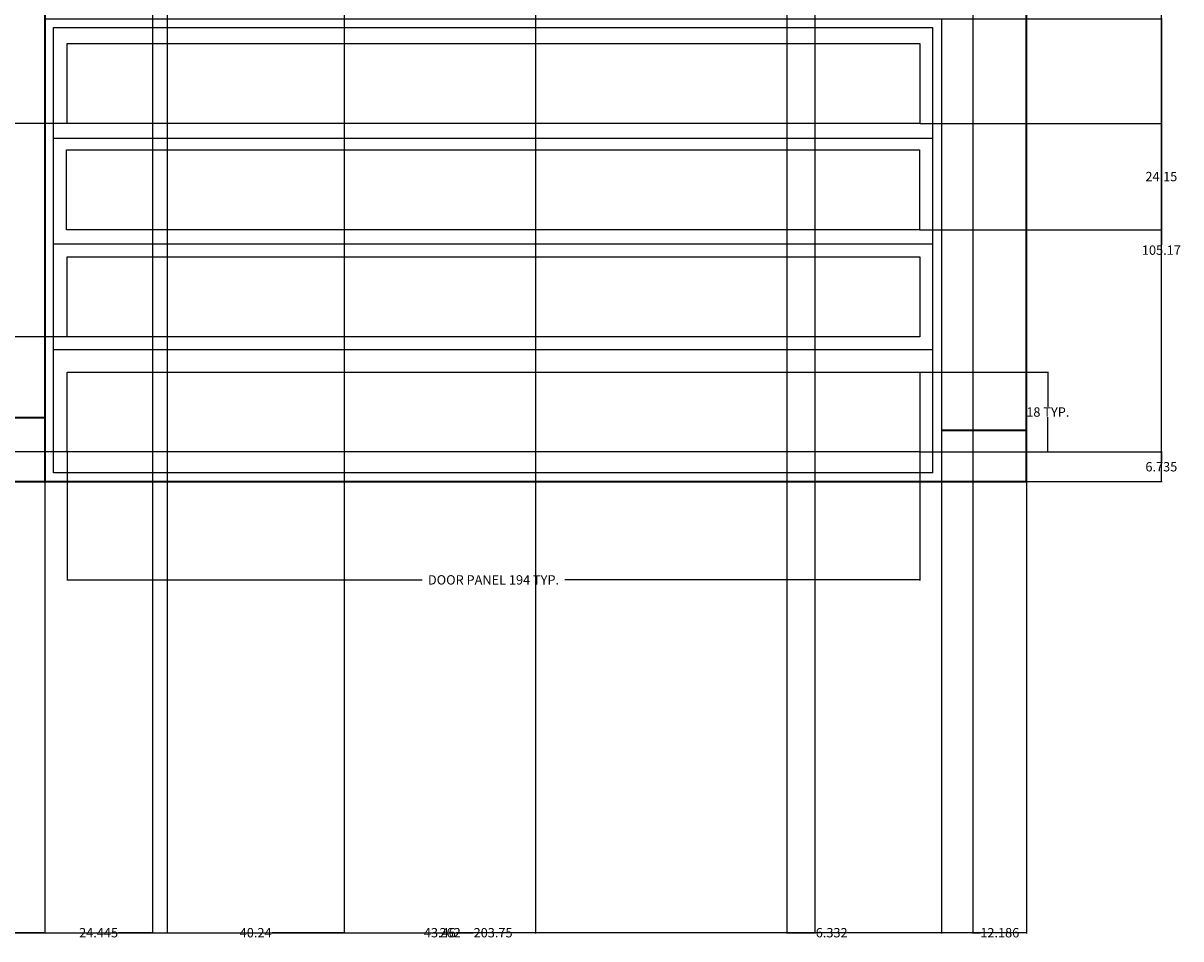
# Model space of a CAD drawing. Units: inches. Extents: x -113 to 379, y 13 to 689.
# Tile 2 of 5: x 116 to 379, y 13 to 221. Entities that reach past the tile are written whole.
import ezdxf

# ---------------------------------------------------------------- set-up
doc = ezdxf.new("R2010")
doc.units = ezdxf.units.IN
doc.header["$MEASUREMENT"] = 0
for name, color, linetype, lineweight in [('A-ANNO-DIMS', 2, 'Continuous', 18), ('A-DOOR', 3, 'Continuous', 25), ('A-WALL', 7, 'Continuous', 35), ('C-TOPO', 8, 'Continuous', 35)]:
    doc.layers.add(name, color=color, linetype=linetype, lineweight=lineweight)
doc.styles.get("Standard").update_dxf_attribs({"font": 'arial.ttf'})
doc.dimstyles.get("Standard").update_dxf_attribs({"dimtxt": 2.125, "dimasz": 0.18, "dimexe": 0.18, "dimexo": 0.0625, "dimgap": 0.09, "dimtad": 0, "dimtih": 1, "dimtoh": 1, "dimdec": 4, "dimzin": 0, "dimdsep": 46, "dimlunit": 4, "dimtxsty": 'Standard', "dimcen": 0.09, "dimadec": 0, "dimazin": 0, "dimtfac": 1, "dimtdec": 4, "dimtofl": 0, "dimtmove": 0, "dimatfit": 3, "dimfxl": 1, "dimtolj": 1, "dimtzin": 0, "dimarcsym": 0})

# ---------------------------------------------------------------- blocks, each defined once
blk = doc.blocks.new('GARAGE-DOOR-PANEL')
blk.add_lwpolyline([(0, 18.13), (193.81, 18.13), (193.81, 0), (0, 0)], close=True)
blk = doc.blocks.new('*D11')
at = {"layer": 'A-ANNO-DIMS', "color": 0, "lineweight": -2, "transparency": 16777216}
for p, q in [((125.81, 123.32), (125.81, 94.13)), ((319.62, 123.32), (319.62, 94.13)), ((125.99, 94.31), (206.54, 94.31)), ((319.44, 94.31), (238.9, 94.31))]:
    blk.add_line(p, q, dxfattribs=at)
at = {"layer": 'A-ANNO-DIMS', "color": 0, "transparency": 16777216}
for points in [[(125.99, 94.34), (125.99, 94.28), (125.81, 94.31)], [(319.44, 94.34), (319.44, 94.28), (319.62, 94.31)]]:
    blk.add_solid(points, dxfattribs=at)
at = {"layer": 'Defpoints', "color": 0, "transparency": 16777216}
for p in [(125.81, 123.39), (319.62, 123.39), (319.62, 94.31)]:
    blk.add_point(p, dxfattribs=at)
at = {"layer": 'A-ANNO-DIMS', "color": 0, "transparency": 16777216, "insert": (222.72, 94.31), "char_height": 2.125, "attachment_point": 5}
blk.add_mtext('\\A1;DOOR PANEL 194 TYP.', dxfattribs=at)
blk = doc.blocks.new('*D12')
at = {"layer": 'A-ANNO-DIMS', "color": 0, "lineweight": -2, "transparency": 16777216}
for p, q in [((319.69, 141.52), (348.88, 141.52)), ((348.7, 141.34), (348.7, 133.63)), ((348.7, 123.57), (348.7, 131.28)), ((319.69, 123.39), (348.88, 123.39))]:
    blk.add_line(p, q, dxfattribs=at)
at = {"layer": 'A-ANNO-DIMS', "color": 0, "transparency": 16777216}
for points in [[(348.67, 141.34), (348.73, 141.34), (348.7, 141.52)], [(348.67, 123.57), (348.73, 123.57), (348.7, 123.39)]]:
    blk.add_solid(points, dxfattribs=at)
at = {"layer": 'Defpoints', "color": 0, "transparency": 16777216}
for p in [(319.62, 141.52), (348.7, 141.52), (319.62, 123.39)]:
    blk.add_point(p, dxfattribs=at)
at = {"layer": 'A-ANNO-DIMS', "color": 0, "transparency": 16777216, "insert": (348.7, 132.45), "char_height": 2.125, "attachment_point": 5}
blk.add_mtext('\\A1;18 TYP.', dxfattribs=at)
blk = doc.blocks.new('*D19')
at = {"layer": 'A-ANNO-DIMS', "color": 0, "lineweight": -2, "transparency": 16777216}
for p, q in [((81.87, 116.59), (81.87, 13.95)), ((343.87, 116.59), (343.87, 13.95)), ((82.05, 14.13), (210.43, 14.13)), ((343.69, 14.13), (215.32, 14.13))]:
    blk.add_line(p, q, dxfattribs=at)
at = {"layer": 'A-ANNO-DIMS', "color": 0, "transparency": 16777216}
for points in [[(82.05, 14.16), (82.05, 14.1), (81.87, 14.13)], [(343.69, 14.16), (343.69, 14.1), (343.87, 14.13)]]:
    blk.add_solid(points, dxfattribs=at)
at = {"layer": 'Defpoints', "color": 0, "transparency": 16777216}
for p in [(81.87, 116.65), (343.87, 116.65), (343.87, 14.13)]:
    blk.add_point(p, dxfattribs=at)
at = {"layer": 'A-ANNO-DIMS', "color": 0, "transparency": 16777216, "insert": (212.87, 14.13), "char_height": 2.125, "attachment_point": 5}
blk.add_mtext('\\A1;262', dxfattribs=at)
blk = doc.blocks.new('*D20')
at = {"layer": 'A-ANNO-DIMS', "color": 0, "lineweight": -2, "transparency": 16777216}
for p, q in [((232.74, 657.3), (374.68, 657.3)), ((374.5, 657.12), (374.5, 388.15)), ((374.5, 116.83), (374.5, 385.8)), ((343.93, 116.65), (374.68, 116.65))]:
    blk.add_line(p, q, dxfattribs=at)
at = {"layer": 'A-ANNO-DIMS', "color": 0, "transparency": 16777216}
for points in [[(374.47, 657.12), (374.53, 657.12), (374.5, 657.3)], [(374.47, 116.83), (374.53, 116.83), (374.5, 116.65)]]:
    blk.add_solid(points, dxfattribs=at)
at = {"layer": 'Defpoints', "color": 0, "transparency": 16777216}
for p in [(232.68, 657.3), (374.5, 657.3), (343.87, 116.65)]:
    blk.add_point(p, dxfattribs=at)
at = {"layer": 'A-ANNO-DIMS', "color": 0, "transparency": 16777216, "insert": (374.5, 386.98), "char_height": 2.125, "attachment_point": 5}
blk.add_mtext('\\A1;540.7', dxfattribs=at)
blk = doc.blocks.new('*D34')
at = {"layer": 'A-ANNO-DIMS', "color": 0, "lineweight": -2, "transparency": 16777216}
for p, q in [((120.75, 116.59), (120.75, 13.95)), ((324.51, 116.59), (324.51, 13.95)), ((120.93, 14.13), (218.1, 14.13)), ((324.33, 14.13), (227.16, 14.13))]:
    blk.add_line(p, q, dxfattribs=at)
at = {"layer": 'A-ANNO-DIMS', "color": 0, "transparency": 16777216}
for points in [[(120.93, 14.16), (120.93, 14.1), (120.75, 14.13)], [(324.33, 14.16), (324.33, 14.1), (324.51, 14.13)]]:
    blk.add_solid(points, dxfattribs=at)
at = {"layer": 'Defpoints', "color": 0, "transparency": 16777216}
for p in [(120.75, 116.65), (324.51, 116.65), (324.51, 14.13)]:
    blk.add_point(p, dxfattribs=at)
at = {"layer": 'A-ANNO-DIMS', "color": 0, "transparency": 16777216, "insert": (222.63, 14.13), "char_height": 2.125, "attachment_point": 5}
blk.add_mtext('\\A1;203.75', dxfattribs=at)
blk = doc.blocks.new('*D35')
at = {"layer": 'A-ANNO-DIMS', "color": 0, "lineweight": -2, "transparency": 16777216}
for p, q in [((324.57, 221.82), (374.68, 221.82)), ((374.5, 221.64), (374.5, 170.41)), ((374.5, 116.83), (374.5, 168.06)), ((324.57, 116.65), (374.68, 116.65))]:
    blk.add_line(p, q, dxfattribs=at)
at = {"layer": 'A-ANNO-DIMS', "color": 0, "transparency": 16777216}
for points in [[(374.47, 221.64), (374.53, 221.64), (374.5, 221.82)], [(374.47, 116.83), (374.53, 116.83), (374.5, 116.65)]]:
    blk.add_solid(points, dxfattribs=at)
at = {"layer": 'Defpoints', "color": 0, "transparency": 16777216}
for p in [(324.51, 221.82), (374.5, 221.82), (324.51, 116.65)]:
    blk.add_point(p, dxfattribs=at)
at = {"layer": 'A-ANNO-DIMS', "color": 0, "transparency": 16777216, "insert": (374.5, 169.24), "char_height": 2.125, "attachment_point": 5}
blk.add_mtext('\\A1;105.17', dxfattribs=at)
blk = doc.blocks.new('*D37')
at = {"layer": 'A-ANNO-DIMS', "color": 0, "lineweight": -2, "transparency": 16777216}
for p, q in [((99.93, 116.59), (99.93, 13.95)), ((120.75, 116.59), (120.75, 13.95)), ((100.11, 14.13), (106.66, 14.13)), ((120.57, 14.13), (114.03, 14.13))]:
    blk.add_line(p, q, dxfattribs=at)
at = {"layer": 'A-ANNO-DIMS', "color": 0, "transparency": 16777216}
for points in [[(100.11, 14.16), (100.11, 14.1), (99.93, 14.13)], [(120.57, 14.16), (120.57, 14.1), (120.75, 14.13)]]:
    blk.add_solid(points, dxfattribs=at)
at = {"layer": 'Defpoints', "color": 0, "transparency": 16777216}
for p in [(99.93, 116.65), (120.75, 116.65), (120.75, 14.13)]:
    blk.add_point(p, dxfattribs=at)
at = {"layer": 'A-ANNO-DIMS', "color": 0, "transparency": 16777216, "insert": (110.34, 14.13), "char_height": 2.125, "attachment_point": 5}
blk.add_mtext('\\A1;20.82', dxfattribs=at)
blk = doc.blocks.new('*D41')
at = {"layer": 'A-ANNO-DIMS', "color": 0, "lineweight": -2, "transparency": 16777216}
for p, q in [((120.75, 286.39), (120.75, 13.95)), ((145.2, 286.39), (145.2, 13.95)), ((120.93, 14.13), (128.45, 14.13)), ((145.02, 14.13), (137.5, 14.13))]:
    blk.add_line(p, q, dxfattribs=at)
at = {"layer": 'A-ANNO-DIMS', "color": 0, "transparency": 16777216}
for points in [[(120.93, 14.16), (120.93, 14.1), (120.75, 14.13)], [(145.02, 14.16), (145.02, 14.1), (145.2, 14.13)]]:
    blk.add_solid(points, dxfattribs=at)
at = {"layer": 'Defpoints', "color": 0, "transparency": 16777216}
for p in [(120.75, 286.45), (145.2, 286.45), (145.2, 14.13)]:
    blk.add_point(p, dxfattribs=at)
at = {"layer": 'A-ANNO-DIMS', "color": 0, "transparency": 16777216, "insert": (132.98, 14.13), "char_height": 2.125, "attachment_point": 5}
blk.add_mtext('\\A1;24.445', dxfattribs=at)
blk = doc.blocks.new('*D44')
at = {"layer": 'A-ANNO-DIMS', "color": 0, "lineweight": -2, "transparency": 16777216}
for p, q in [((331.68, 303.98), (331.68, 13.95)), ((343.87, 260.59), (343.87, 13.95)), ((331.86, 14.13), (333.38, 14.13)), ((343.69, 14.13), (342.18, 14.13))]:
    blk.add_line(p, q, dxfattribs=at)
at = {"layer": 'A-ANNO-DIMS', "color": 0, "transparency": 16777216}
for points in [[(331.86, 14.16), (331.86, 14.1), (331.68, 14.13)], [(343.69, 14.16), (343.69, 14.1), (343.87, 14.13)]]:
    blk.add_solid(points, dxfattribs=at)
at = {"layer": 'Defpoints', "color": 0, "transparency": 16777216}
for p in [(331.68, 304.04), (343.87, 260.65), (343.87, 14.13)]:
    blk.add_point(p, dxfattribs=at)
at = {"layer": 'A-ANNO-DIMS', "color": 0, "transparency": 16777216, "insert": (337.78, 14.13), "char_height": 2.125, "attachment_point": 5}
blk.add_mtext('\\A1;12.186', dxfattribs=at)
blk = doc.blocks.new('*D46')
at = {"layer": 'A-ANNO-DIMS', "color": 0, "lineweight": -2, "transparency": 16777216}
for p, q in [((295.73, 303.98), (295.73, 13.95)), ((289.4, 260.59), (289.4, 13.95)), ((289.58, 14.13), (295.55, 14.13)), ((295.73, 14.13), (295.91, 14.13))]:
    blk.add_line(p, q, dxfattribs=at)
at = {"layer": 'A-ANNO-DIMS', "color": 0, "transparency": 16777216}
for points in [[(289.58, 14.16), (289.58, 14.1), (289.4, 14.13)], [(295.55, 14.16), (295.55, 14.1), (295.73, 14.13)]]:
    blk.add_solid(points, dxfattribs=at)
at = {"layer": 'Defpoints', "color": 0, "transparency": 16777216}
for p in [(295.73, 304.04), (289.4, 260.65), (295.73, 14.13)]:
    blk.add_point(p, dxfattribs=at)
at = {"layer": 'A-ANNO-DIMS', "color": 0, "transparency": 16777216, "insert": (299.58, 14.13), "char_height": 2.125, "attachment_point": 5}
blk.add_mtext('\\A1;6.332', dxfattribs=at)
blk = doc.blocks.new('*D53')
at = {"layer": 'A-ANNO-DIMS', "color": 0, "lineweight": -2, "transparency": 16777216}
for p, q in [((125.75, 198.04), (-108.66, 198.04)), ((-108.48, 197.86), (-108.48, 174.97)), ((-108.48, 149.74), (-108.48, 172.62)), ((125.75, 149.56), (-108.66, 149.56))]:
    blk.add_line(p, q, dxfattribs=at)
at = {"layer": 'A-ANNO-DIMS', "color": 0, "transparency": 16777216}
for points in [[(-108.51, 197.86), (-108.45, 197.86), (-108.48, 198.04)], [(-108.51, 149.74), (-108.45, 149.74), (-108.48, 149.56)]]:
    blk.add_solid(points, dxfattribs=at)
at = {"layer": 'Defpoints', "color": 0, "transparency": 16777216}
for p in [(125.81, 198.04), (-108.48, 149.56), (125.81, 149.56)]:
    blk.add_point(p, dxfattribs=at)
at = {"layer": 'A-ANNO-DIMS', "color": 0, "transparency": 16777216, "insert": (-108.48, 173.8), "char_height": 2.125, "attachment_point": 5}
blk.add_mtext('\\A1;48.47', dxfattribs=at)
blk = doc.blocks.new('*D54')
at = {"layer": 'A-ANNO-DIMS', "color": 0, "lineweight": -2, "transparency": 16777216}
for p, q in [((125.75, 149.56), (-108.66, 149.56)), ((-108.48, 149.38), (-108.48, 137.65)), ((-108.48, 123.57), (-108.48, 135.3)), ((125.75, 123.39), (-108.66, 123.39))]:
    blk.add_line(p, q, dxfattribs=at)
at = {"layer": 'A-ANNO-DIMS', "color": 0, "transparency": 16777216}
for points in [[(-108.51, 149.38), (-108.45, 149.38), (-108.48, 149.56)], [(-108.51, 123.57), (-108.45, 123.57), (-108.48, 123.39)]]:
    blk.add_solid(points, dxfattribs=at)
at = {"layer": 'Defpoints', "color": 0, "transparency": 16777216}
for p in [(125.81, 149.56), (-108.48, 123.39), (125.81, 123.39)]:
    blk.add_point(p, dxfattribs=at)
at = {"layer": 'A-ANNO-DIMS', "color": 0, "transparency": 16777216, "insert": (-108.48, 136.47), "char_height": 2.125, "attachment_point": 5}
blk.add_mtext('\\A1;26.177', dxfattribs=at)
blk = doc.blocks.new('*D55')
at = {"layer": 'A-ANNO-DIMS', "color": 0, "lineweight": -2, "transparency": 16777216}
for p, q in [((319.69, 198.04), (374.68, 198.04)), ((374.5, 197.86), (374.5, 187.13)), ((374.5, 174.06), (374.5, 184.78)), ((319.6, 173.88), (374.68, 173.88))]:
    blk.add_line(p, q, dxfattribs=at)
at = {"layer": 'A-ANNO-DIMS', "color": 0, "transparency": 16777216}
for points in [[(374.47, 197.86), (374.53, 197.86), (374.5, 198.04)], [(374.47, 174.06), (374.53, 174.06), (374.5, 173.88)]]:
    blk.add_solid(points, dxfattribs=at)
at = {"layer": 'Defpoints', "color": 0, "transparency": 16777216}
for p in [(319.62, 198.04), (319.54, 173.88), (374.5, 173.88)]:
    blk.add_point(p, dxfattribs=at)
at = {"layer": 'A-ANNO-DIMS', "color": 0, "transparency": 16777216, "insert": (374.5, 185.96), "char_height": 2.125, "attachment_point": 5}
blk.add_mtext('\\A1;24.15', dxfattribs=at)
blk = doc.blocks.new('*D56')
at = {"layer": 'A-ANNO-DIMS', "color": 0, "lineweight": -2, "transparency": 16777216}
for p, q in [((148.55, 291.91), (148.55, 13.95)), ((188.79, 291.91), (188.79, 13.95)), ((148.73, 14.13), (164.96, 14.13)), ((188.61, 14.13), (172.39, 14.13))]:
    blk.add_line(p, q, dxfattribs=at)
at = {"layer": 'A-ANNO-DIMS', "color": 0, "transparency": 16777216}
for points in [[(148.73, 14.16), (148.73, 14.1), (148.55, 14.13)], [(188.61, 14.16), (188.61, 14.1), (188.79, 14.13)]]:
    blk.add_solid(points, dxfattribs=at)
at = {"layer": 'Defpoints', "color": 0, "transparency": 16777216}
for p in [(148.55, 291.98), (188.79, 291.98), (188.79, 14.13)]:
    blk.add_point(p, dxfattribs=at)
at = {"layer": 'A-ANNO-DIMS', "color": 0, "transparency": 16777216, "insert": (168.67, 14.13), "char_height": 2.125, "attachment_point": 5}
blk.add_mtext('\\A1;40.24', dxfattribs=at)
blk = doc.blocks.new('*D57')
at = {"layer": 'A-ANNO-DIMS', "color": 0, "lineweight": -2, "transparency": 16777216}
for p, q in [((188.79, 291.91), (188.79, 13.95)), ((232.25, 291.91), (232.25, 13.95)), ((188.97, 14.13), (206.81, 14.13)), ((232.07, 14.13), (214.24, 14.13))]:
    blk.add_line(p, q, dxfattribs=at)
at = {"layer": 'A-ANNO-DIMS', "color": 0, "transparency": 16777216}
for points in [[(188.97, 14.16), (188.97, 14.1), (188.79, 14.13)], [(232.07, 14.16), (232.07, 14.1), (232.25, 14.13)]]:
    blk.add_solid(points, dxfattribs=at)
at = {"layer": 'Defpoints', "color": 0, "transparency": 16777216}
for p in [(188.79, 291.98), (232.25, 291.98), (232.25, 14.13)]:
    blk.add_point(p, dxfattribs=at)
at = {"layer": 'A-ANNO-DIMS', "color": 0, "transparency": 16777216, "insert": (210.52, 14.13), "char_height": 2.125, "attachment_point": 5}
blk.add_mtext('\\A1;43.46', dxfattribs=at)
blk = doc.blocks.new('*D70')
at = {"layer": 'A-ANNO-DIMS', "color": 0, "lineweight": -2, "transparency": 16777216}
for p, q in [((319.69, 123.39), (374.68, 123.39)), ((374.5, 123.21), (374.5, 121.19)), ((374.5, 116.83), (374.5, 118.84)), ((324.57, 116.65), (374.68, 116.65))]:
    blk.add_line(p, q, dxfattribs=at)
at = {"layer": 'A-ANNO-DIMS', "color": 0, "transparency": 16777216}
for points in [[(374.47, 123.21), (374.53, 123.21), (374.5, 123.39)], [(374.47, 116.83), (374.53, 116.83), (374.5, 116.65)]]:
    blk.add_solid(points, dxfattribs=at)
at = {"layer": 'Defpoints', "color": 0, "transparency": 16777216}
for p in [(319.62, 123.39), (374.5, 123.39), (324.51, 116.65)]:
    blk.add_point(p, dxfattribs=at)
at = {"layer": 'A-ANNO-DIMS', "color": 0, "transparency": 16777216, "insert": (374.5, 120.02), "char_height": 2.125, "attachment_point": 5}
blk.add_mtext('\\A1;6.735', dxfattribs=at)

msp = doc.modelspace()

# ---------------------------------------------------------------- linework, layer by layer
at = {"layer": 'A-DOOR'}
for p, q in [((122.7533, 194.6775), (322.5073, 194.6775)), ((122.7533, 170.6775), (322.5073, 170.6775)), ((122.7533, 146.6775), (322.5073, 146.6775))]:
    msp.add_line(p, q, dxfattribs=at)
for points in [[(120.7533, 221.8228), (324.5073, 221.8228), (324.5073, 116.6509), (120.7533, 116.6509)], [(122.7533, 219.8228), (322.5073, 219.8228), (322.5073, 118.6509), (122.7533, 118.6509)]]:
    msp.add_lwpolyline(points, close=True, dxfattribs=at)
at = {"layer": 'A-WALL'}
for p, q in [((120.7533, 260.6509), (120.7533, 116.6509)), ((343.8693, 116.6509), (343.8693, 260.6509)), ((74.6887, 131.237), (120.7533, 131.237)), ((324.5073, 128.3599), (343.8693, 128.3599))]:
    msp.add_line(p, q, dxfattribs=at)
at = {"layer": 'C-TOPO'}
msp.add_line((-14.3304, 116.6509), (343.8693, 116.6509), dxfattribs=at)

# ---------------------------------------------------------------- block references
at = {"layer": 'A-DOOR'}
for p in [(125.8084, 198.0351), (125.7228, 173.8839), (125.8084, 149.5623), (125.8084, 123.3856)]:
    msp.add_blockref('GARAGE-DOOR-PANEL', p, dxfattribs=at)

# ---------------------------------------------------------------- dimensions: what is measured, and where the dimension line sits
at = {"layer": 'A-ANNO-DIMS'}
for base, p1, p2, override, picture, middle in [((374.5043, 657.3014), (343.8693, 116.6509), (232.6797, 657.3014), {"dimdec": 1, "dimlfac": 1, "dimrnd": 0, "dimzin": 0, "dimdsep": 46, "dimlunit": 2}, '*D20', (374.5043, 386.9762)), ((374.5043, 221.8228), (324.5073, 116.6509), (324.5073, 221.8228), {"dimdec": 2, "dimlfac": 1, "dimrnd": 0, "dimzin": 0, "dimdsep": 46, "dimlunit": 2}, '*D35', (374.5043, 169.2369)), ((-108.4772, 149.5623), (125.8084, 198.0351), (125.8084, 149.5623), {"dimdec": 2, "dimlfac": 1, "dimrnd": 0, "dimzin": 0, "dimdsep": 46, "dimlunit": 2}, '*D53', (-108.4772, 173.7987)), ((374.5043, 173.8839), (319.6234, 198.0351), (319.5378, 173.8839), {"dimdec": 2, "dimlfac": 1, "dimrnd": 0, "dimzin": 0, "dimdsep": 46, "dimlunit": 2}, '*D55', (374.5043, 185.9595)), ((-108.4772, 123.3856), (125.8084, 149.5623), (125.8084, 123.3856), {"dimdec": 3, "dimlfac": 1, "dimrnd": 0, "dimzin": 0, "dimdsep": 46, "dimlunit": 2}, '*D54', (-108.4772, 136.4739)), ((374.5043, 123.3856), (324.5073, 116.6509), (319.6234, 123.3856), {"dimdec": 3, "dimlfac": 1, "dimrnd": 0, "dimzin": 0, "dimdsep": 46, "dimlunit": 2}, '*D70', (374.5043, 120.0182))]:
    dim = msp.add_linear_dim(base=base, p1=p1, p2=p2, angle=90, dimstyle='Standard', override=override, dxfattribs=at)
    dim.commit()
    dim.dimension.update_dxf_attribs({"geometry": picture, "text_midpoint": middle})
for base, p1, p2, override, picture, middle in [((295.728, 14.1289), (289.3958, 260.6509), (295.728, 304.0445), {"dimdec": 3, "dimlfac": 1, "dimrnd": 0, "dimzin": 0, "dimdsep": 46, "dimlunit": 2}, '*D46', (299.5783, 14.1289)), ((343.8693, 14.1289), (331.6831, 304.0445), (343.8693, 260.6509), {"dimdec": 3, "dimlfac": 1, "dimrnd": 0, "dimzin": 0, "dimdsep": 46, "dimlunit": 2}, '*D44', (337.7762, 14.1289)), ((188.7939, 14.1289), (148.5524, 291.9762), (188.7939, 291.9762), {"dimdec": 2, "dimlfac": 1, "dimrnd": 0, "dimzin": 0, "dimdsep": 46, "dimlunit": 2}, '*D56', (168.6732, 14.1289)), ((232.2544, 14.1289), (188.7939, 291.9762), (232.2544, 291.9762), {"dimdec": 2, "dimlfac": 1, "dimrnd": 0, "dimzin": 0, "dimdsep": 46, "dimlunit": 2}, '*D57', (210.5242, 14.1289)), ((145.1985, 14.1289), (120.7533, 286.4497), (145.1985, 286.4497), {"dimdec": 3, "dimlfac": 1, "dimrnd": 0, "dimzin": 0, "dimdsep": 46, "dimlunit": 2}, '*D41', (132.9759, 14.1289)), ((343.8693, 14.1289), (81.8721, 116.6509), (343.8693, 116.6509), {"dimdec": 0, "dimlfac": 1, "dimrnd": 0, "dimzin": 0, "dimdsep": 46, "dimlunit": 2}, '*D19', (212.8707, 14.1289)), ((120.7533, 14.1289), (99.9328, 116.6509), (120.7533, 116.6509), {"dimdec": 2, "dimlfac": 1, "dimrnd": 0, "dimzin": 0, "dimdsep": 46, "dimlunit": 2}, '*D37', (110.3431, 14.1289)), ((324.5073, 14.1289), (120.7533, 116.6509), (324.5073, 116.6509), {"dimdec": 2, "dimlfac": 1, "dimrnd": 0, "dimzin": 0, "dimdsep": 46, "dimlunit": 2}, '*D34', (222.6303, 14.1289))]:
    dim = msp.add_linear_dim(base=base, p1=p1, p2=p2, dimstyle='Standard', override=override, dxfattribs=at)
    dim.commit()
    dim.dimension.update_dxf_attribs({"geometry": picture, "text_midpoint": middle})
dim = msp.add_linear_dim(base=(348.6956, 141.5153), p1=(319.6234, 123.3856), p2=(319.6234, 141.5153), angle=90, text='<> TYP.', dimstyle='Standard', override={"dimdec": 0, "dimlfac": 1, "dimrnd": 0, "dimzin": 0, "dimdsep": 46, "dimlunit": 2}, dxfattribs=at)
dim.commit()
dim.dimension.update_dxf_attribs({"geometry": '*D12', "text_midpoint": (348.6956, 132.4504)})
dim = msp.add_linear_dim(base=(319.6234, 94.3133), p1=(125.8084, 123.3856), p2=(319.6234, 123.3856), text='DOOR PANEL <> TYP.', dimstyle='Standard', override={"dimdec": 0, "dimlfac": 1, "dimrnd": 0, "dimzin": 0, "dimdsep": 46, "dimlunit": 2}, dxfattribs=at)
dim.commit()
dim.dimension.update_dxf_attribs({"geometry": '*D11', "text_midpoint": (222.7159, 94.3133)})

doc.saveas('drawing.dxf')
